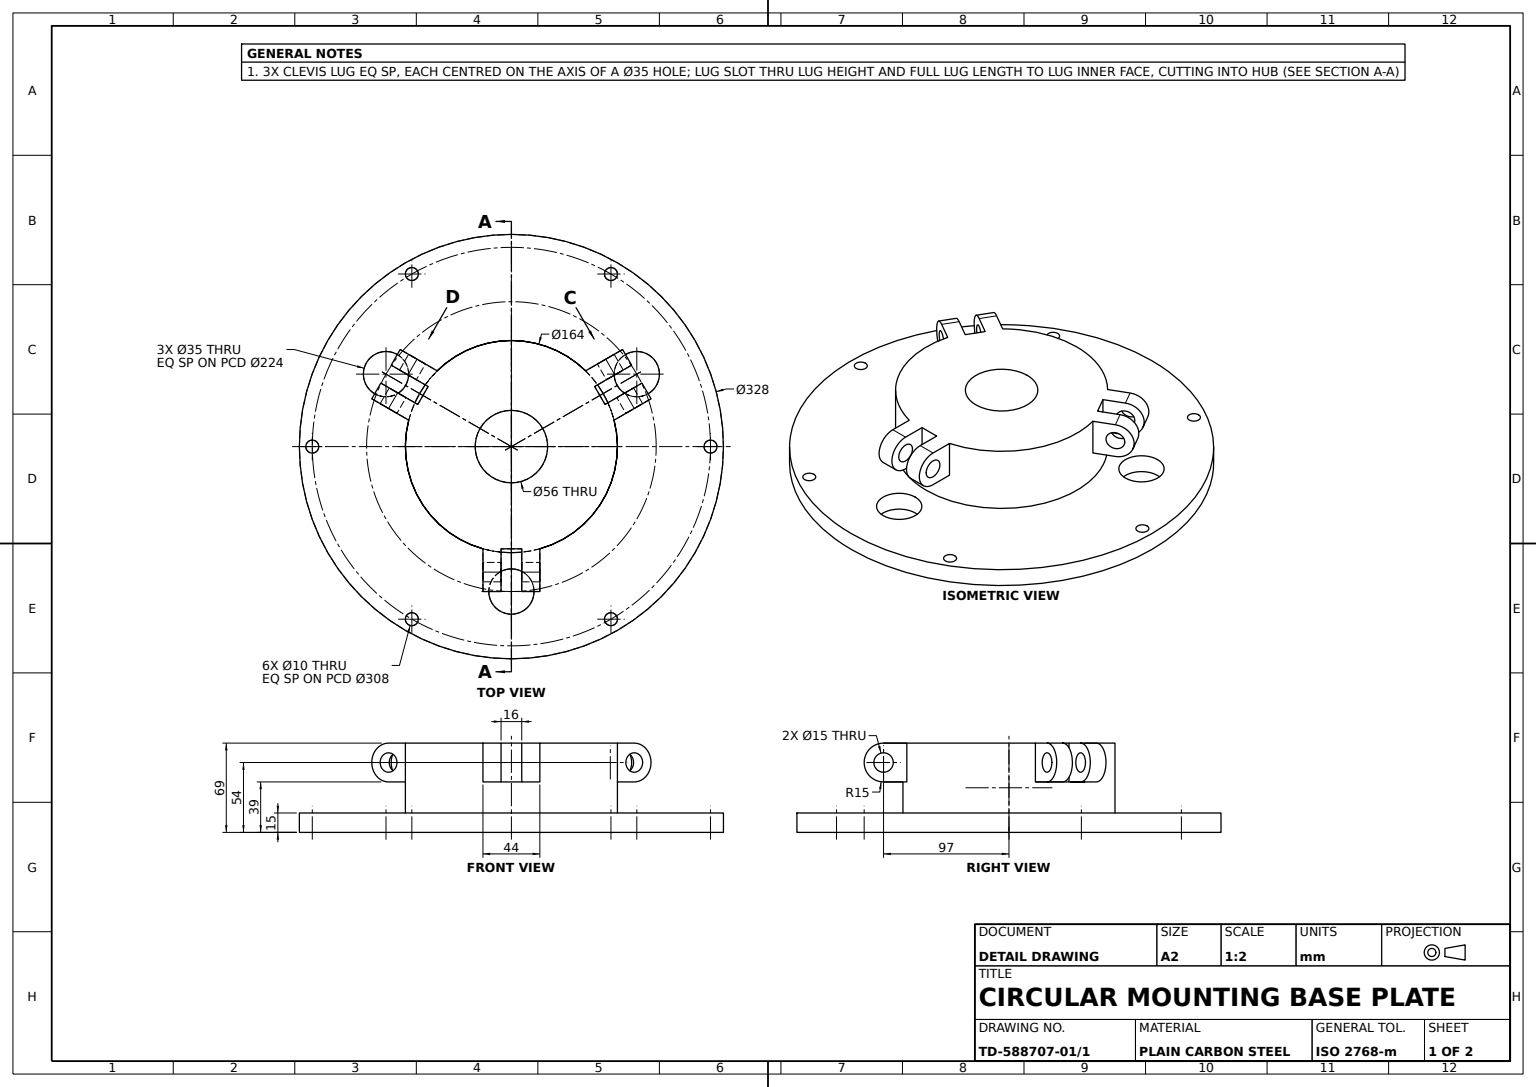
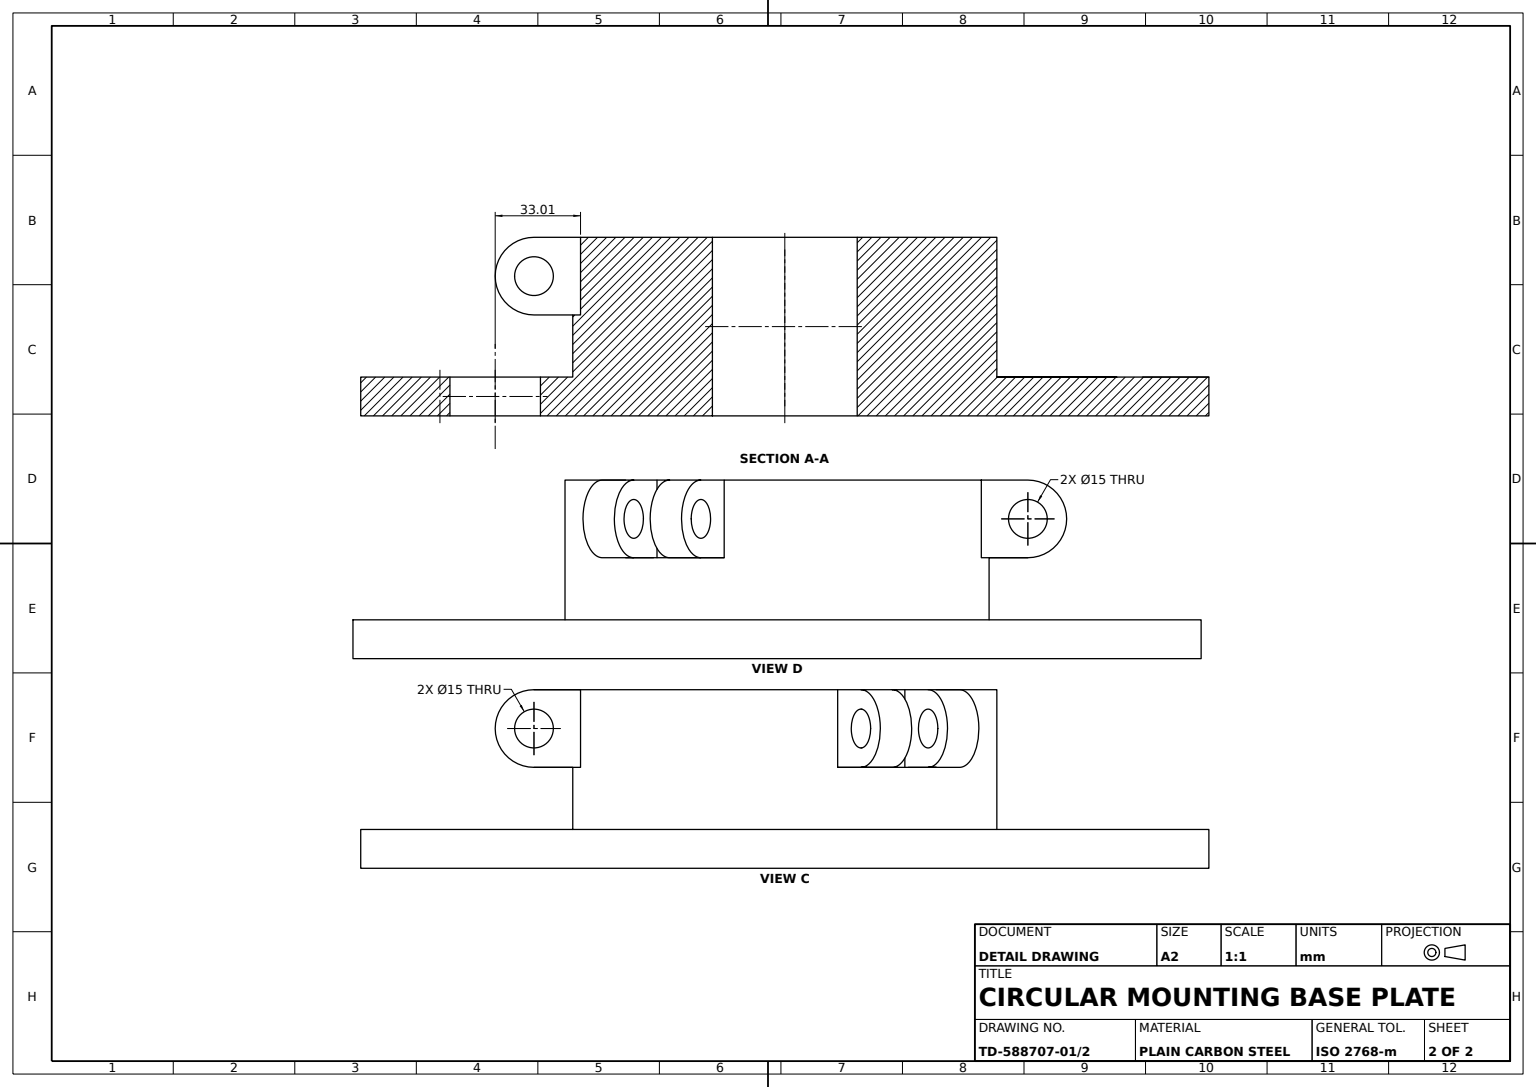
from build123d import *

# Parameters (mm, degrees)
BASE_DISC_SKETCH_328_R            = 164
BASE_DISC_328X15_DEPTH            = 15
HUB_SKETCH_164_R                  = 82
HUB_164X54_DEPTH                  = 54
CENTRE_BORE_SKETCH_56_R           = 28
CENTRE_BORE_56_DEPTH              = 242.97727166
CLEVIS_LUG_PROFILE_SKETCH_R       = 7.5
CLEVIS_LUG_DEPTH                  = 22
CLEVIS_SLOT_30_DEPTH              = 30
CLEVIS_LUG_PATTERN_3X_COUNT       = 3
LARGE_HOLE_SKETCH_35_R            = 17.5
LARGE_HOLE_35_DEPTH               = 239.134415824
LARGE_HOLE_PATTERN_3X_35_COUNT    = 3
MOUNTING_HOLE_SKETCH_10_R         = 5
MOUNTING_HOLE_10_DEPTH            = 242.97727166
MOUNTING_HOLE_PATTERN_6X_10_COUNT = 6


with BuildPart() as part:
    # Base Disc Sketch Ø328 → Base Disc Ø328x15 (new body)
    with BuildSketch(Plane(origin=(0, 0, 0), x_dir=(1, 0, 0), z_dir=(0, 1, 0))):
        with Locations(Location((0, 0, 0), (0, 0, 270))):
            Circle(BASE_DISC_SKETCH_328_R)
    extrude(amount=BASE_DISC_328X15_DEPTH)

    # Hub Sketch Ø164 → Hub Ø164x54 (add)
    with BuildSketch(Plane(origin=(0, 15, 0), x_dir=(1, 0, 0), z_dir=(0, 1, 0))):
        with Locations(Location((0, 0, 0), (0, 0, 270))):
            Circle(HUB_SKETCH_164_R)
    extrude(amount=HUB_164X54_DEPTH)

    # Centre Bore Sketch Ø56 → Centre Bore Ø56 (cut, through all)
    with BuildSketch(Plane(origin=(0, 69, 0), x_dir=(1, 0, 0), z_dir=(0, 1, 0))):
        with Locations(Location((0, 0, 0), (0, 0, 270))):
            Circle(CENTRE_BORE_SKETCH_56_R)
    extrude(amount=-CENTRE_BORE_56_DEPTH, mode=Mode.SUBTRACT)

    # Clevis Lug Profile Sketch → Clevis Lug (add, symmetric)
    with BuildSketch(Plane(origin=(0, 0, 0), x_dir=(0, 0, -1), z_dir=(1, 0, 0))):
        with BuildLine():
            Line((-97, 69), (-69.408237338, 69))
            Line((-69.408237338, 69), (-69.408237338, 39))
            Line((-69.408237338, 39), (-97, 39))
            ThreePointArc((-97, 39), (-112, 54), (-97, 69))
        make_face()
        with Locations((-97, 54)):
            Circle(CLEVIS_LUG_PROFILE_SKETCH_R, mode=Mode.SUBTRACT)
    clevis_lug = extrude(amount=CLEVIS_LUG_DEPTH, both=True)

    # Clevis Slot Profile Sketch → Clevis Slot 30 (cut)
    with BuildSketch(Plane(origin=(0, 69, 0), x_dir=(1, 0, 0), z_dir=(0, 1, 0))):
        Polygon((0, -112), (-8, -112), (-8, -78.993670633), (8, -78.993670633), (8, -112), align=None)
    clevis_slot_30 = extrude(amount=-CLEVIS_SLOT_30_DEPTH, mode=Mode.SUBTRACT)

    # Clevis Lug Pattern 3x: Clevis Lug, Clevis Slot 30 ×3 about axis
    clevis_lug_pattern_3x_axis = Axis((0, 0, 0), (0, 1, 0))
    add([clevis_lug.rotate(clevis_lug_pattern_3x_axis, i * 360 / CLEVIS_LUG_PATTERN_3X_COUNT) for i in range(1, CLEVIS_LUG_PATTERN_3X_COUNT)])
    add([clevis_slot_30.rotate(clevis_lug_pattern_3x_axis, i * 360 / CLEVIS_LUG_PATTERN_3X_COUNT) for i in range(1, CLEVIS_LUG_PATTERN_3X_COUNT)], mode=Mode.SUBTRACT)

    # Large Hole Sketch Ø35 → Large Hole Ø35 (cut, through all)
    with BuildSketch(Plane(origin=(0, 15, 0), x_dir=(1, 0, 0), z_dir=(0, 1, 0))):
        with Locations(Location((0, -112, 0), (0, 0, 270))):
            Circle(LARGE_HOLE_SKETCH_35_R)
    large_hole_35 = extrude(amount=-LARGE_HOLE_35_DEPTH, mode=Mode.SUBTRACT)

    # Large Hole Pattern 3xØ35: Large Hole Ø35 ×3 about axis
    large_hole_pattern_3x_35_axis = Axis((0, 0, 0), (0, 1, 0))
    for i in range(1, LARGE_HOLE_PATTERN_3X_35_COUNT):
        add(large_hole_35.rotate(large_hole_pattern_3x_35_axis, i * 360 / LARGE_HOLE_PATTERN_3X_35_COUNT), mode=Mode.SUBTRACT)

    # Mounting Hole Sketch Ø10 → Mounting Hole Ø10 (cut, through all)
    with BuildSketch(Plane(origin=(0, 69, 0), x_dir=(1, 0, 0), z_dir=(0, 1, 0))):
        with Locations(Location((-154, 0, 0), (0, 0, 270))):
            Circle(MOUNTING_HOLE_SKETCH_10_R)
    mounting_hole_10 = extrude(amount=-MOUNTING_HOLE_10_DEPTH, mode=Mode.SUBTRACT)

    # Mounting Hole Pattern 6xØ10: Mounting Hole Ø10 ×6 about axis
    mounting_hole_pattern_6x_10_axis = Axis((0, 0, 0), (0, 1, 0))
    for i in range(1, MOUNTING_HOLE_PATTERN_6X_10_COUNT):
        add(mounting_hole_10.rotate(mounting_hole_pattern_6x_10_axis, i * 360 / MOUNTING_HOLE_PATTERN_6X_10_COUNT), mode=Mode.SUBTRACT)


solid = part.part
